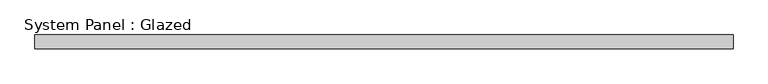
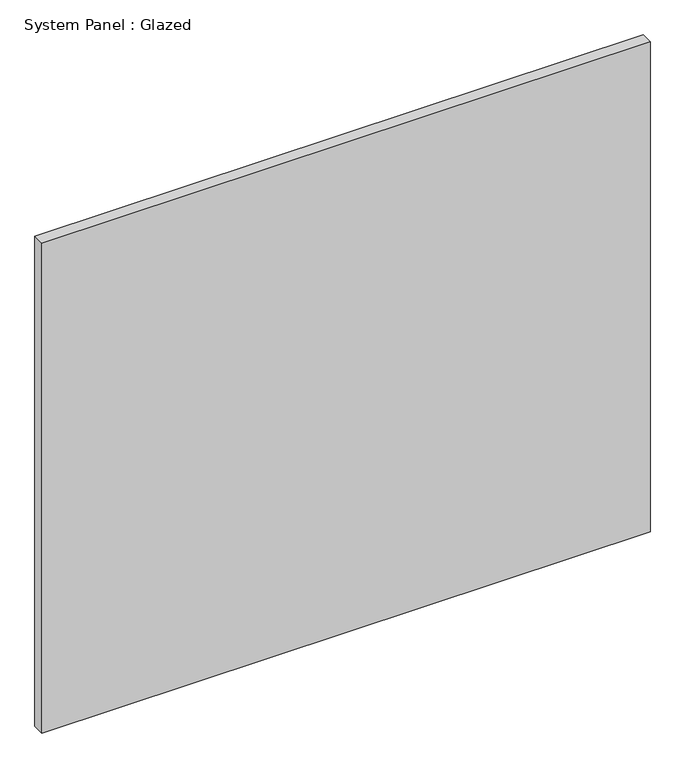
"""IFC4 building model written with IfcOpenShell, lengths in millimetres: plate geometry, System Panel : Glazed."""

from ifc_helpers import new_model, si_unit, origin, origin_with_axes, place, context, project, spatial, polyline, outline, extrude, source, transform, mapped, element, save


def system_panel_glazed_87944ff9(model_context):
    return source(origin(), model_context, "Body", "SweptSolid", [
        extrude(outline(polyline([(641.35, 19.05), (-641.35, 19.05), (-641.35, 44.45), (641.35, 44.45), (641.35, 19.05)])), origin_with_axes(), (0.0, 0.0, 1.0), 1092.2),
    ])


if __name__ == "__main__":
    model = new_model("IFC4")
    model_context = context("Model", 3, world=origin())
    ifc_project = project(units=[si_unit("LENGTHUNIT", "METRE", prefix="MILLI")], contexts=[model_context])
    site = spatial("IfcSite", under=ifc_project)
    building = spatial("IfcBuilding", under=site)
    placement = place(None, origin())
    system_panel_glazed_shape = system_panel_glazed_87944ff9(model_context)
    element("IfcPlate", 1, ObjectType="System Panel : Glazed", at=placement, inside=building, context=model_context, shape_type="MappedRepresentation", body=[
        mapped(system_panel_glazed_shape, transform((0.0, 0.0, 0.0), x_axis=(1.0, 0.0, 0.0), y_axis=(0.0, 1.0, 0.0), z_axis=(0.0, 0.0, 1.0))),
    ])
    save(model, "model.ifc")

# Revit data of these elements
# Type "System Panel : Glazed"
#   Construction Type Id = "GSP4R"
#   Analytic Construction = "1/8 in Pilkington single glazing"
#   Visual Light Transmittance = 0.9
#   Solar Heat Gain Coefficient = 0.86
#   Heat Transfer Coefficient (U) = 1.18115 BTU/(h·ft²·°F)
#   Define Thermal Properties by = 1
# Element 1 (IfcPlate, "System Panel : Glazed")
#   Materials on its faces: "Glass"
# Materials
#   "Glass": class "Glass", colour RGB 0 128 192, transparency 0.75, Description = "Soda Lime Glass", Cost = 0
